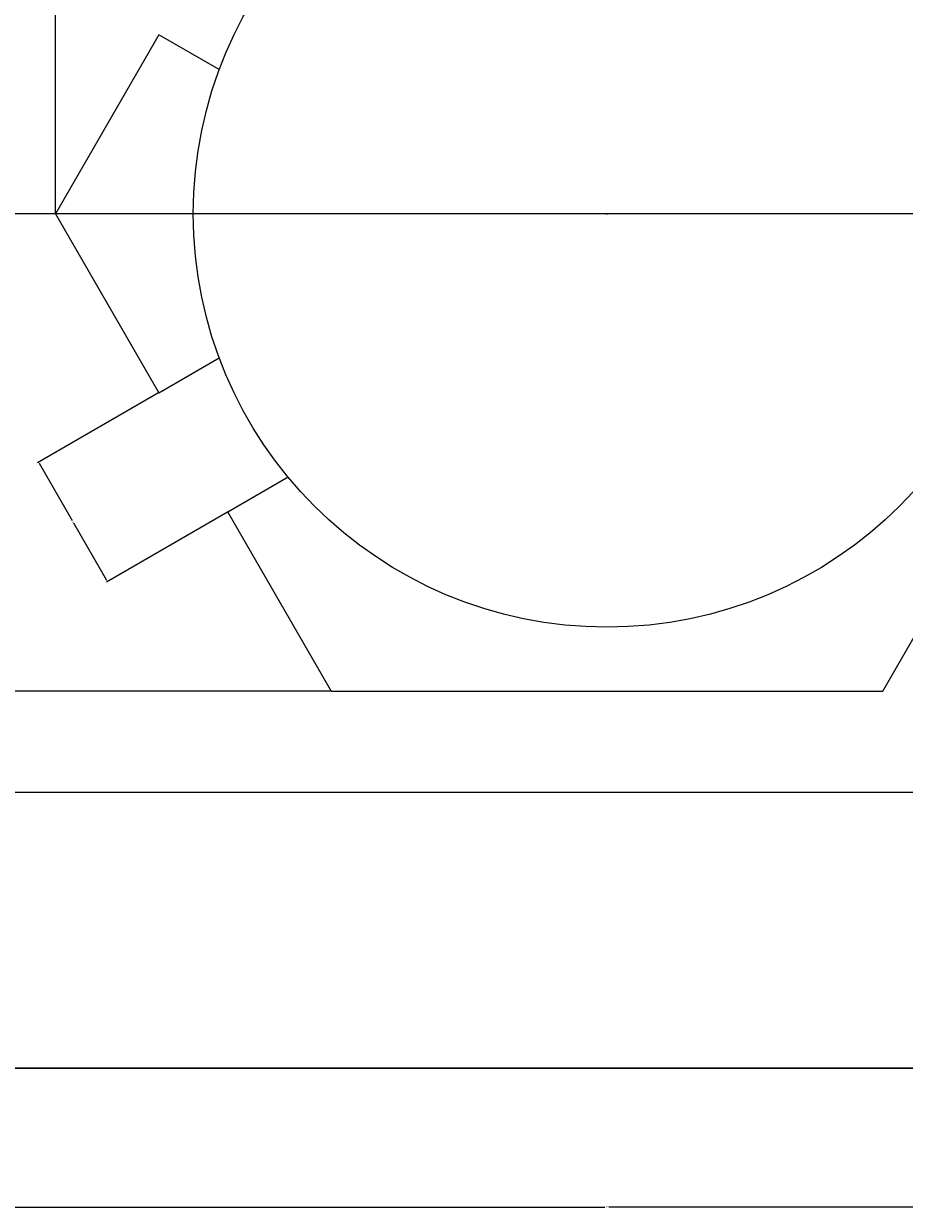
# Model space of a CAD drawing. Units: inches. Extents: x 1095 to 1408, y -20 to 240.
# Tile 4 of 8: x 1167 to 1294, y -20 to 152. Entities that reach past the tile are written whole.
import ezdxf

# ---------------------------------------------------------------- set-up
doc = ezdxf.new("R2010")
doc.units = ezdxf.units.IN
doc.header["$MEASUREMENT"] = 0
doc.layers.add('M-CONS', color=8, linetype='Continuous', lineweight=18)
doc.layers.add('M-DIMS', color=2, linetype='Continuous', lineweight=18)
doc.styles.get("Standard").update_dxf_attribs({"font": 'arial.ttf'})
doc.dimstyles.get("Standard").update_dxf_attribs({"dimtxt": 0.18, "dimasz": 0.18, "dimexe": 0.18, "dimexo": 0.0625, "dimgap": 0.09, "dimtad": 0, "dimtih": 1, "dimtoh": 1, "dimdec": 4, "dimzin": 0, "dimdsep": 46, "dimtxsty": 'Standard', "dimcen": 0.09, "dimadec": 0, "dimazin": 0, "dimtfac": 1, "dimtdec": 4, "dimtofl": 0, "dimtmove": 0, "dimatfit": 3, "dimfxl": 1, "dimtolj": 1, "dimtzin": 0, "dimarcsym": 0})

# ---------------------------------------------------------------- blocks, each defined once
blk = doc.blocks.new('*D1')
at = {"layer": 'Defpoints', "color": 0, "transparency": 16777216}
for p in [(1115.18, 0), (1387.18, 0), (1387.18, -20.15)]:
    blk.add_point(p, dxfattribs=at)
at = {"layer": 'M-DIMS', "color": 0, "lineweight": -2, "transparency": 16777216}
for p, q in [((1115.18, -0.06), (1115.18, -20.33)), ((1387.18, -0.06), (1387.18, -20.33)), ((1115.36, -20.15), (1250.89, -20.15)), ((1387, -20.15), (1251.47, -20.15))]:
    blk.add_line(p, q, dxfattribs=at)
at = {"layer": 'M-DIMS', "color": 0, "transparency": 16777216}
for points in [[(1115.36, -20.12), (1115.36, -20.18), (1115.18, -20.15)], [(1387, -20.12), (1387, -20.18), (1387.18, -20.15)]]:
    blk.add_solid(points, dxfattribs=at)
at = {"layer": 'M-DIMS', "color": 0, "transparency": 16777216, "insert": (1251.18, -20.15), "char_height": 0.18, "attachment_point": 5}
blk.add_mtext('\\A1;272', dxfattribs=at)
blk = doc.blocks.new('*D8')
at = {"layer": 'Defpoints', "color": 0, "transparency": 16777216}
for p in [(1095.03, 124), (1387.18, 124), (1365.18, 40)]:
    blk.add_point(p, dxfattribs=at)
at = {"layer": 'M-DIMS', "color": 0, "lineweight": -2, "transparency": 16777216}
for p, q in [((1387.12, 124), (1094.85, 124)), ((1095.03, 123.82), (1095.03, 82.18)), ((1095.03, 40.18), (1095.03, 81.82)), ((1365.12, 40), (1094.85, 40))]:
    blk.add_line(p, q, dxfattribs=at)
at = {"layer": 'M-DIMS', "color": 0, "transparency": 16777216}
for points in [[(1095, 123.82), (1095.06, 123.82), (1095.03, 124)], [(1095, 40.18), (1095.06, 40.18), (1095.03, 40)]]:
    blk.add_solid(points, dxfattribs=at)
at = {"layer": 'M-DIMS', "color": 0, "transparency": 16777216, "insert": (1095.03, 82), "char_height": 0.18, "attachment_point": 5}
blk.add_mtext('\\A1;84', dxfattribs=at)
blk = doc.blocks.new('*D9')
at = {"layer": 'Defpoints', "color": 0, "transparency": 16777216}
for p in [(1331.18, 239.75), (1171.18, 124), (1331.18, 124)]:
    blk.add_point(p, dxfattribs=at)
at = {"layer": 'M-DIMS', "color": 0, "lineweight": -2, "transparency": 16777216}
for p, q in [((1171.18, 124.06), (1171.18, 239.93)), ((1171.36, 239.75), (1250.9, 239.75)), ((1331, 239.75), (1251.46, 239.75)), ((1331.18, 124.06), (1331.18, 239.93))]:
    blk.add_line(p, q, dxfattribs=at)
at = {"layer": 'M-DIMS', "color": 0, "transparency": 16777216}
for points in [[(1171.36, 239.78), (1171.36, 239.72), (1171.18, 239.75)], [(1331, 239.78), (1331, 239.72), (1331.18, 239.75)]]:
    blk.add_solid(points, dxfattribs=at)
at = {"layer": 'M-DIMS', "color": 0, "transparency": 16777216, "insert": (1251.18, 239.75), "char_height": 0.18, "attachment_point": 5}
blk.add_mtext('\\A1;160', dxfattribs=at)
blk = doc.blocks.new('*D10')
at = {"layer": 'Defpoints', "color": 0, "transparency": 16777216}
for p in [(1095.03, 193.28), (1211.18, 193.28), (1211.18, 54.72)]:
    blk.add_point(p, dxfattribs=at)
at = {"layer": 'M-DIMS', "color": 0, "lineweight": -2, "transparency": 16777216}
for p, q in [((1211.12, 193.28), (1094.85, 193.28)), ((1095.03, 193.1), (1095.03, 124.18)), ((1095.03, 54.9), (1095.03, 123.82)), ((1211.12, 54.72), (1094.85, 54.72))]:
    blk.add_line(p, q, dxfattribs=at)
at = {"layer": 'M-DIMS', "color": 0, "transparency": 16777216}
for points in [[(1095, 193.1), (1095.06, 193.1), (1095.03, 193.28)], [(1095, 54.9), (1095.06, 54.9), (1095.03, 54.72)]]:
    blk.add_solid(points, dxfattribs=at)
at = {"layer": 'M-DIMS', "color": 0, "transparency": 16777216, "insert": (1095.03, 124), "char_height": 0.18, "attachment_point": 5}
blk.add_mtext('\\A1;138.56', dxfattribs=at)
blk = doc.blocks.new('*D12')
at = {"layer": 'Defpoints', "color": 0, "transparency": 16777216}
for p in [(1186.18, 98.02), (1168.73, 87.94), (1196.18, 80.7)]:
    blk.add_point(p, dxfattribs=at)
at = {"layer": 'M-DIMS', "color": 0, "lineweight": -2, "transparency": 16777216}
for p, q in [((1186.13, 97.99), (1168.58, 87.85)), ((1168.82, 87.79), (1173.63, 79.47)), ((1178.64, 70.78), (1173.84, 79.1)), ((1196.13, 80.67), (1178.58, 70.53))]:
    blk.add_line(p, q, dxfattribs=at)
at = {"layer": 'M-DIMS', "color": 0, "transparency": 16777216}
for points in [[(1168.85, 87.8), (1168.8, 87.77), (1168.73, 87.94)], [(1178.67, 70.79), (1178.62, 70.76), (1178.73, 70.62)]]:
    blk.add_solid(points, dxfattribs=at)
at = {"layer": 'M-DIMS', "color": 0, "transparency": 16777216, "insert": (1173.73, 79.28), "char_height": 0.18, "attachment_point": 5}
blk.add_mtext('\\A1;20', dxfattribs=at)
blk = doc.blocks.new('*D18')
at = {"layer": 'Defpoints', "color": 0, "transparency": 16777216}
for p in [(1251.18, 184), (1251.18, 64)]:
    blk.add_point(p, dxfattribs=at)
at = {"layer": 'M-DIMS', "color": 0, "lineweight": -2, "transparency": 16777216}
for p, q in [((1251.36, 220), (1251.18, 220)), ((1251.18, 220), (1251.18, 184.18)), ((1251.09, 124), (1251.27, 124)), ((1251.18, 123.91), (1251.18, 124.09))]:
    blk.add_line(p, q, dxfattribs=at)
at = {"layer": 'M-DIMS', "color": 0, "transparency": 16777216}
blk.add_solid([(1251.15, 184.18), (1251.21, 184.18), (1251.18, 184)], dxfattribs=at)
at = {"layer": 'M-DIMS', "color": 0, "transparency": 16777216, "insert": (1251.75, 220), "char_height": 0.18, "attachment_point": 5}
blk.add_mtext('\\A1;∅120', dxfattribs=at)

msp = doc.modelspace()

# ---------------------------------------------------------------- linework, layer by layer
at = {"layer": 'M-CONS', "extrusion": (0, -1, 0)}
for p, q in [((1115.184, 0, 357.783), (1387.184, 0, 357.783)), ((1383.184, 0, 377.783), (1119.184, 0, 377.783))]:
    msp.add_line(p, q, dxfattribs=at)
at = {"layer": 'M-CONS', "elevation": 377.783}
for points in [[(1194.949, 144.92), (1186.184, 149.981), (1171.184, 124), (1186.184, 98.019), (1194.949, 103.08)], [(1204.949, 85.759), (1196.184, 80.699), (1211.184, 54.718), (1291.184, 54.718), (1306.184, 80.699), (1297.418, 85.759)]]:
    msp.add_lwpolyline(points, dxfattribs=at)
at = {"layer": 'M-CONS'}
msp.add_circle((1251.184, 124, 377.783), 60, dxfattribs=at)

# ---------------------------------------------------------------- dimensions: what is measured, and where the dimension line sits
at = {"layer": 'M-DIMS'}
for base, p1, p2, picture, middle in [((1331.184, 239.75), (1171.184, 124), (1331.184, 124), '*D9', (1251.184, 239.75)), ((1387.184, -20.15), (1115.184, 0), (1387.184, 0), '*D1', (1251.184, -20.15))]:
    dim = msp.add_linear_dim(base=base, p1=p1, p2=p2, dimstyle='Standard', override={"dimdec": 0, "dimlfac": 1, "dimrnd": 0, "dimzin": 0, "dimdsep": 46, "dimlunit": 2}, dxfattribs=at)
    dim.commit()
    dim.dimension.update_dxf_attribs({"geometry": picture, "text_midpoint": middle})
dim = msp.add_diameter_dim_2p(p1=(1251.183, 64), p2=(1251.184, 184), dimstyle='Standard', override={"dimdec": 0, "dimlfac": 1, "dimrnd": 0, "dimzin": 0, "dimdsep": 46, "dimlunit": 2}, dxfattribs=at)
dim.commit()
dim.dimension.update_dxf_attribs({"geometry": '*D18', "text_midpoint": (1251.751, 220), "dimtype": 163})
for base, p1, p2, angle, override, picture, middle in [((1095.034, 193.282), (1211.184, 54.718), (1211.184, 193.282), 90, {"dimdec": 2, "dimlfac": 1, "dimrnd": 0, "dimzin": 0, "dimdsep": 46, "dimlunit": 2}, '*D10', (1095.034, 124)), ((1095.034, 124), (1365.184, 40), (1387.184, 124), 90, {"dimdec": 0, "dimlfac": 1, "dimrnd": 0, "dimzin": 0, "dimdsep": 46, "dimlunit": 2}, '*D8', (1095.034, 82)), ((1168.733, 87.944), (1196.184, 80.699), (1186.184, 98.019), 120, {"dimdec": 0, "dimlfac": 1, "dimrnd": 0, "dimzin": 0, "dimdsep": 46, "dimlunit": 2}, '*D12', (1173.733, 79.284))]:
    dim = msp.add_linear_dim(base=base, p1=p1, p2=p2, angle=angle, dimstyle='Standard', override=override, dxfattribs=at)
    dim.commit()
    dim.dimension.update_dxf_attribs({"geometry": picture, "text_midpoint": middle})

doc.saveas('drawing.dxf')
